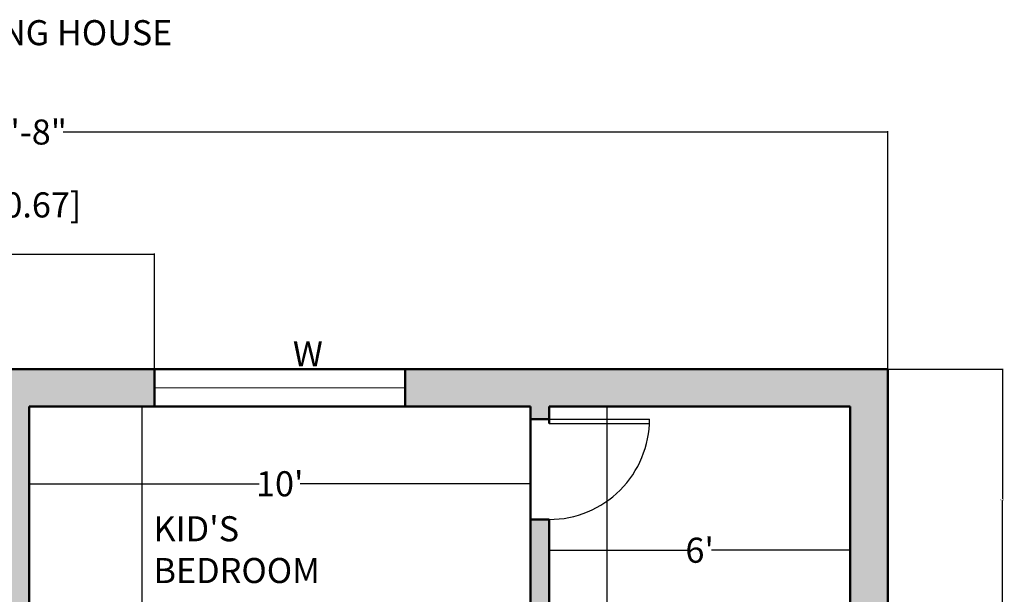
# Model space of a CAD drawing. Units: inches. Extents: x -22 to 470, y -437 to 97.
# Tile 9 of 9: x 235 to 470, y -41 to 97. Entities that reach past the tile are written whole.
import ezdxf

# ---------------------------------------------------------------- set-up
doc = ezdxf.new("R2010")
doc.units = ezdxf.units.IN
doc.header["$MEASUREMENT"] = 0
for name, color, linetype, lineweight in [('A-ANNO-DIMS', 2, 'Continuous', 18), ('A-ANNO-TEXT', 7, 'Continuous', 18), ('A-AREA-IDEN', 7, 'Continuous', 25), ('A-DOOR', 4, 'Continuous', 25), ('A-GLAZ', 4, 'Continuous', 18), ('A-WALL', 7, 'Continuous', 50), ('A-WALL-PATT', 8, 'Continuous', 13)]:
    doc.layers.add(name, color=color, linetype=linetype, lineweight=lineweight)
doc.styles.get("Standard").update_dxf_attribs({"font": 'arial.ttf'})
doc.dimstyles.get("Standard").update_dxf_attribs({"dimtxt": 0.18, "dimasz": 0.18, "dimexe": 0.18, "dimexo": 0.0625, "dimgap": 0.09, "dimtad": 0, "dimtih": 1, "dimtoh": 1, "dimdec": 0, "dimzin": 0, "dimdsep": 46, "dimlunit": 3, "dimtxsty": 'Standard', "dimcen": 0.09, "dimadec": 0, "dimazin": 0, "dimtfac": 1, "dimtdec": 0, "dimtofl": 0, "dimtmove": 0, "dimatfit": 3, "dimfxl": 1, "dimtolj": 1, "dimtzin": 0, "dimarcsym": 0})

# ---------------------------------------------------------------- blocks, each defined once
blk = doc.blocks.new('*D2')
at = {"layer": 'A-ANNO-DIMS', "color": 0, "lineweight": -2, "transparency": 16777216}
for p, q in [((26.92, 13.31), (26.92, 70.17)), ((27.1, 69.99), (224.28, 69.99)), ((442.24, 69.99), (245.07, 69.99)), ((442.42, 13.31), (442.42, 70.17))]:
    blk.add_line(p, q, dxfattribs=at)
at = {"layer": 'A-ANNO-DIMS', "color": 0, "transparency": 16777216}
for points in [[(27.1, 70.02), (27.1, 69.96), (26.92, 69.99)], [(442.24, 70.02), (442.24, 69.96), (442.42, 69.99)]]:
    blk.add_solid(points, dxfattribs=at)
at = {"layer": 'Defpoints', "color": 0, "transparency": 16777216}
for p in [(442.42, 69.99), (26.92, 13.24), (442.42, 13.24)]:
    blk.add_point(p, dxfattribs=at)
at = {"layer": 'A-ANNO-DIMS', "color": 0, "transparency": 16777216, "insert": (234.67, 69.99), "char_height": 6, "attachment_point": 5}
blk.add_mtext('\\A1;34\'-8"', dxfattribs=at)
blk = doc.blocks.new('*D8')
at = {"layer": 'A-ANNO-DIMS', "color": 0, "lineweight": -2, "transparency": 16777216}
for p, q in [((236.92, -14.15), (236.92, -14.04)), ((356.92, -14.15), (356.92, -14.04)), ((237.1, -14.22), (292.02, -14.22)), ((356.74, -14.22), (301.82, -14.22))]:
    blk.add_line(p, q, dxfattribs=at)
at = {"layer": 'A-ANNO-DIMS', "color": 0, "transparency": 16777216}
for points in [[(237.1, -14.19), (237.1, -14.25), (236.92, -14.22)], [(356.74, -14.19), (356.74, -14.25), (356.92, -14.22)]]:
    blk.add_solid(points, dxfattribs=at)
at = {"layer": 'Defpoints', "color": 0, "transparency": 16777216}
for p in [(236.92, -14.22), (356.92, -14.22), (356.92, -14.22)]:
    blk.add_point(p, dxfattribs=at)
at = {"layer": 'A-ANNO-DIMS', "color": 0, "transparency": 16777216, "insert": (296.92, -14.22), "char_height": 6, "attachment_point": 5}
blk.add_mtext("\\A1;10'", dxfattribs=at)
blk = doc.blocks.new('*D9')
at = {"layer": 'A-ANNO-DIMS', "color": 0, "lineweight": -2, "transparency": 16777216}
for p, q in [((263.92, 4.06), (263.92, -52.6)), ((263.98, 4.24), (264.1, 4.24)), ((263.92, -115.58), (263.92, -58.91)), ((263.98, -115.76), (264.1, -115.76))]:
    blk.add_line(p, q, dxfattribs=at)
at = {"layer": 'A-ANNO-DIMS', "color": 0, "transparency": 16777216}
for points in [[(263.89, 4.06), (263.95, 4.06), (263.92, 4.24)], [(263.89, -115.58), (263.95, -115.58), (263.92, -115.76)]]:
    blk.add_solid(points, dxfattribs=at)
at = {"layer": 'Defpoints', "color": 0, "transparency": 16777216}
for p in [(263.92, 4.24), (263.92, -115.76), (263.92, -115.76)]:
    blk.add_point(p, dxfattribs=at)
at = {"layer": 'A-ANNO-DIMS', "color": 0, "transparency": 16777216, "insert": (263.92, -55.76), "char_height": 6, "attachment_point": 5}
blk.add_mtext("\\A1;10'", dxfattribs=at)
blk = doc.blocks.new('*D10')
at = {"layer": 'A-ANNO-DIMS', "color": 0, "lineweight": -2, "transparency": 16777216}
for p, q in [((361.42, -31.79), (361.42, -29.95)), ((361.6, -30.13), (394.55, -30.13)), ((433.24, -30.13), (400.29, -30.13)), ((433.42, -31.79), (433.42, -29.95))]:
    blk.add_line(p, q, dxfattribs=at)
at = {"layer": 'A-ANNO-DIMS', "color": 0, "transparency": 16777216}
for points in [[(361.6, -30.1), (361.6, -30.16), (361.42, -30.13)], [(433.24, -30.1), (433.24, -30.16), (433.42, -30.13)]]:
    blk.add_solid(points, dxfattribs=at)
at = {"layer": 'Defpoints', "color": 0, "transparency": 16777216}
for p in [(433.42, -30.13), (361.42, -31.86), (433.42, -31.86)]:
    blk.add_point(p, dxfattribs=at)
at = {"layer": 'A-ANNO-DIMS', "color": 0, "transparency": 16777216, "insert": (397.42, -30.13), "char_height": 6, "attachment_point": 5}
blk.add_mtext("\\A1;6'", dxfattribs=at)
blk = doc.blocks.new('*D11')
at = {"layer": 'A-ANNO-DIMS', "color": 0, "lineweight": -2, "transparency": 16777216}
for p, q in [((386.2, 4.24), (375.02, 4.24)), ((375.2, 4.06), (375.2, -52.6)), ((375.2, -115.58), (375.2, -58.91)), ((386.2, -115.76), (375.02, -115.76))]:
    blk.add_line(p, q, dxfattribs=at)
at = {"layer": 'A-ANNO-DIMS', "color": 0, "transparency": 16777216}
for points in [[(375.17, 4.06), (375.23, 4.06), (375.2, 4.24)], [(375.17, -115.58), (375.23, -115.58), (375.2, -115.76)]]:
    blk.add_solid(points, dxfattribs=at)
at = {"layer": 'Defpoints', "color": 0, "transparency": 16777216}
for p in [(386.26, 4.24), (375.2, -115.76), (386.26, -115.76)]:
    blk.add_point(p, dxfattribs=at)
at = {"layer": 'A-ANNO-DIMS', "color": 0, "transparency": 16777216, "insert": (375.2, -55.76), "char_height": 6, "attachment_point": 5}
blk.add_mtext("\\A1;10'", dxfattribs=at)
blk = doc.blocks.new('DOOR-SWING-24')
for p, q in [((23, 24), (23, 0)), ((24, 24), (24, 0))]:
    blk.add_line(p, q)
blk.add_arc((24, 24), 24, 180, 270)
blk = doc.blocks.new('WINDOW-60-SASH')
for p, q in [((0, 9), (60, 9)), ((0, 4.5), (60, 4.5)), ((60, 0), (0, 0))]:
    blk.add_line(p, q)
blk = doc.blocks.new('*D66')
at = {"layer": 'A-ANNO-DIMS', "color": 0, "lineweight": -2, "transparency": 16777216}
for p, q in [((190.42, 13.31), (190.42, 40.87)), ((190.6, 40.69), (228.13, 40.69)), ((266.74, 40.69), (229.21, 40.69)), ((266.92, 13.31), (266.92, 40.87))]:
    blk.add_line(p, q, dxfattribs=at)
at = {"layer": 'A-ANNO-DIMS', "color": 0, "transparency": 16777216}
for points in [[(190.6, 40.72), (190.6, 40.66), (190.42, 40.69)], [(266.74, 40.72), (266.74, 40.66), (266.92, 40.69)]]:
    blk.add_solid(points, dxfattribs=at)
at = {"layer": 'Defpoints', "color": 0, "transparency": 16777216}
for p in [(266.92, 40.69), (190.42, 13.24), (266.92, 13.24)]:
    blk.add_point(p, dxfattribs=at)
at = {"layer": 'A-ANNO-DIMS', "color": 0, "transparency": 16777216, "insert": (228.67, 40.69), "char_height": 0.18, "attachment_point": 5}
blk.add_mtext('\\A1;6\'-4 1/2"', dxfattribs=at)
blk = doc.blocks.new('*D70')
at = {"layer": 'A-ANNO-DIMS', "color": 0, "lineweight": -2, "transparency": 16777216}
for p, q in [((442.48, 13.24), (470.05, 13.24)), ((469.87, 13.06), (469.87, -17.88)), ((469.87, -49.2), (469.87, -18.25)), ((442.48, -49.38), (470.05, -49.38))]:
    blk.add_line(p, q, dxfattribs=at)
at = {"layer": 'A-ANNO-DIMS', "color": 0, "transparency": 16777216}
for points in [[(469.84, 13.06), (469.9, 13.06), (469.87, 13.24)], [(469.84, -49.2), (469.9, -49.2), (469.87, -49.38)]]:
    blk.add_solid(points, dxfattribs=at)
at = {"layer": 'Defpoints', "color": 0, "transparency": 16777216}
for p in [(442.42, 13.24), (442.42, -49.38), (469.87, -49.38)]:
    blk.add_point(p, dxfattribs=at)
at = {"layer": 'A-ANNO-DIMS', "color": 0, "transparency": 16777216, "insert": (469.87, -18.07), "char_height": 0.18, "attachment_point": 5}
blk.add_mtext('\\A1;5\'-2 1/2"', dxfattribs=at)

msp = doc.modelspace()

# ---------------------------------------------------------------- hatches: boundary and pattern name
at = {"layer": 'A-WALL-PATT'}
h = msp.add_hatch(color=256, dxfattribs=at)
h.dxf.hatch_style = 1
h.paths.add_polyline_path([(130.42, 13.24), (26.92, 13.24), (26.92, -43.76), (35.92, -43.76), (35.92, 4.24), (83.92, 4.24), (83.92, 1.24), (88.42, 1.24), (88.42, 4.24), (130.42, 4.24)])
h.paths.add_polyline_path([(266.92, 13.24), (190.42, 13.24), (190.42, 4.24), (232.42, 4.24), (232.42, -115.76), (229.42, -115.76), (229.42, -120.26), (239.92, -120.26), (239.92, -115.76), (236.92, -115.76), (236.92, 4.24), (266.92, 4.24)])
h.paths.add_polyline_path([(442.42, 13.24), (326.92, 13.24), (326.92, 4.24), (356.92, 4.24), (356.92, 1.24), (361.42, 1.24), (361.42, 4.24), (433.42, 4.24), (433.42, -49.38), (442.42, -49.38)])
h.paths.add_polyline_path([(442.42, -73.38), (433.42, -73.38), (433.42, -115.76), (361.42, -115.76), (361.42, -22.76), (356.92, -22.76), (356.92, -115.76), (263.92, -115.76), (263.92, -120.26), (332.92, -120.26), (332.92, -123.26), (337.42, -123.26), (337.42, -120.26), (433.42, -120.26), (433.42, -148.49), (442.42, -148.49)])
h.paths.add_polyline_path([(205.42, -115.76), (88.42, -115.76), (88.42, -22.76), (83.92, -22.76), (83.92, -115.76), (35.92, -115.76), (35.92, -67.76), (26.92, -67.76), (26.92, -126.26), (35.92, -126.26), (35.92, -120.26), (205.42, -120.26)])
h.paths.add_polyline_path([(35.92, -196.76), (168.92, -196.76), (168.92, -192.26), (35.92, -192.26), (35.92, -186.26), (26.92, -186.26), (26.92, -224.25), (35.92, -224.25)])
h.paths.add_polyline_path([(35.92, -284.25), (26.92, -284.25), (26.92, -397.76), (53.92, -397.76), (53.92, -388.76), (35.92, -388.76)])
h.paths.add_polyline_path([(142.42, -388.76), (136.42, -388.76), (136.42, -316.76), (181.42, -316.76), (181.42, -312.26), (136.42, -312.26), (136.42, -303.75), (131.92, -303.75), (131.92, -388.76), (113.92, -388.76), (113.92, -397.76), (142.42, -397.76)])
h.paths.add_polyline_path([(218.92, -388.76), (212.92, -388.76), (212.92, -312.26), (205.42, -312.26), (205.42, -316.76), (208.42, -316.76), (208.42, -388.76), (202.42, -388.76), (202.42, -397.76), (218.92, -397.76)])
h.paths.add_polyline_path([(306.75, -388.76), (289.42, -388.76), (289.42, -316.76), (284.92, -316.76), (284.92, -388.76), (278.92, -388.76), (278.92, -397.76), (306.75, -397.76)])
h.paths.add_polyline_path([(391.42, -388.76), (366.75, -388.76), (366.75, -397.76), (391.42, -397.76)], flags=17)
h.paths.add_polyline_path([(442.42, -172.49), (433.42, -172.49), (433.42, -192.26), (337.42, -192.26), (337.42, -147.26), (332.92, -147.26), (332.92, -196.76), (433.42, -196.76), (433.42, -388.76), (427.42, -388.76), (427.42, -397.76), (442.42, -397.76)])

# ---------------------------------------------------------------- linework, layer by layer
at = {"layer": 'A-WALL'}
for p, q in [((26.92, 13.24), (442.42, 13.24)), ((266.92, 4.24), (266.92, 13.24)), ((326.92, 13.24), (326.92, 4.24)), ((442.42, 13.24), (442.42, -397.76)), ((236.92, 4.24), (236.92, -115.76)), ((236.92, 4.24), (356.92, 4.24)), ((356.92, 4.24), (356.92, -115.76)), ((361.42, 4.24), (361.42, 0.24)), ((361.42, 4.24), (433.42, 4.24)), ((433.42, 4.24), (433.42, -115.76)), ((361.42, 1.24), (356.92, 1.24)), ((361.42, -22.76), (356.92, -22.76)), ((361.42, -22.76), (361.42, -115.76))]:
    msp.add_line(p, q, dxfattribs=at)

# ---------------------------------------------------------------- block references
at = {"layer": 'A-DOOR', "rotation": 89.99999999999984}
msp.add_blockref('DOOR-SWING-24', (385.42, -22.76), dxfattribs=at)
at = {"layer": 'A-GLAZ'}
msp.add_blockref('WINDOW-60-SASH', (266.92, 4.24), dxfattribs=at)

# ---------------------------------------------------------------- texts
at = {"layer": 'A-ANNO-DIMS', "insert": (223.46, 55.54), "char_height": 6, "attachment_point": 1}
msp.add_mtext_dynamic_manual_height_columns('[10.67]', width=2.641, gutter_width=1, heights=[0], dxfattribs=at)
at = {"layer": 'A-ANNO-TEXT', "char_height": 6, "attachment_point": 1}
for s, insert in [('EAST FACING HOUSE', (191.66, 96.78)), ('W', (300.05, 19.91))]:
    msp.add_mtext(s, dxfattribs=dict(at, insert=insert))
at = {"layer": 'A-AREA-IDEN', "insert": (266.71, -21.99), "char_height": 6, "attachment_point": 1}
msp.add_mtext("KID'S \\PBEDROOM", dxfattribs=at)

# ---------------------------------------------------------------- dimensions: what is measured, and where the dimension line sits
at = {"layer": 'A-ANNO-DIMS'}
for base, p1, p2, override, picture, middle in [((442.42161427, 69.98621919), (26.92161427, 13.24363331), (442.42161427, 13.24363331), {"dimtxt": 6, "dimclrd": 0, "dimclre": 0, "dimclrt": 0}, '*D2', (234.67161427, 69.98621919)), ((266.92, 40.69), (190.42, 13.24), (266.92, 13.24), {"dimdec": 1, "dimlfac": 1, "dimrnd": 0, "dimzin": 1, "dimdsep": 46, "dimlunit": 4, "dimfrac": 2}, '*D66', (228.67, 40.69)), ((356.92, -14.22), (236.92, -14.22), (356.92, -14.22), {"dimtxt": 6, "dimclrd": 0, "dimclre": 0, "dimclrt": 0}, '*D8', (296.92, -14.22)), ((433.42, -30.13), (361.42, -31.86), (433.42, -31.86), {"dimtxt": 6, "dimclrd": 0, "dimclre": 0, "dimclrt": 0}, '*D10', (397.42, -30.13))]:
    dim = msp.add_linear_dim(base=base, p1=p1, p2=p2, dimstyle='Standard', override=override, dxfattribs=at)
    dim.commit()
    dim.dimension.update_dxf_attribs({"geometry": picture, "text_midpoint": middle})
for base, p1, p2, override, picture, middle in [((469.87, -49.38), (442.42, 13.24), (442.42, -49.38), {"dimdec": 1, "dimlfac": 1, "dimrnd": 0, "dimzin": 1, "dimdsep": 46, "dimlunit": 4, "dimfrac": 2}, '*D70', (469.87, -18.07)), ((263.92, -115.76), (263.92, 4.24), (263.92, -115.76), {"dimtxt": 6, "dimclrd": 0, "dimclre": 0, "dimclrt": 0}, '*D9', (263.92, -55.76)), ((375.2, -115.76), (386.26, 4.24), (386.26, -115.76), {"dimtxt": 6, "dimclrd": 0, "dimclre": 0, "dimclrt": 0}, '*D11', (375.2, -55.76))]:
    dim = msp.add_linear_dim(base=base, p1=p1, p2=p2, angle=90, dimstyle='Standard', override=override, dxfattribs=at)
    dim.commit()
    dim.dimension.update_dxf_attribs({"geometry": picture, "text_midpoint": middle})

doc.saveas('drawing.dxf')
